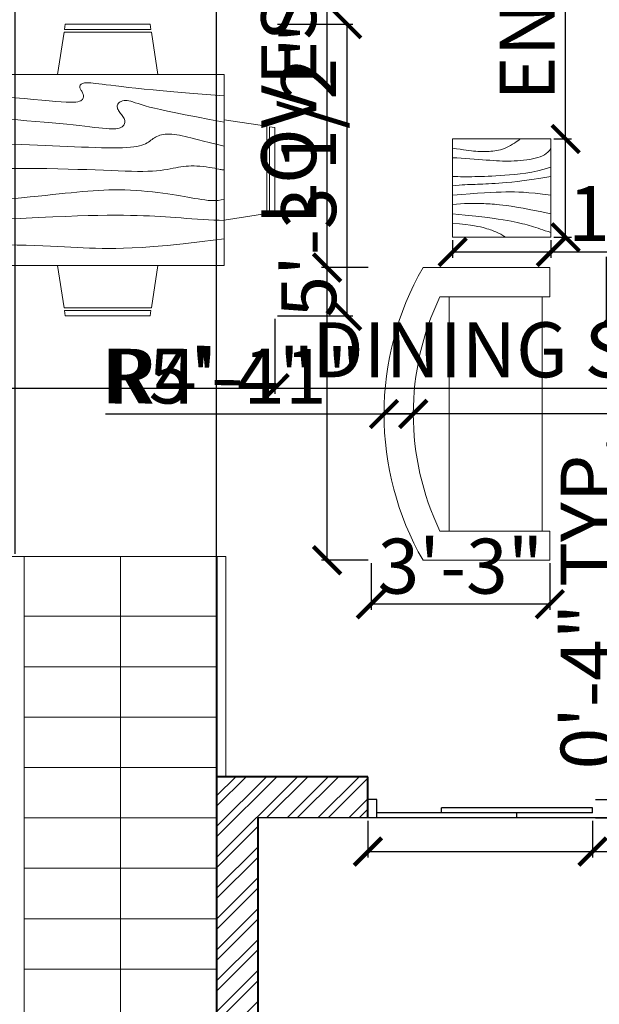
# Model space of a CAD drawing. Units: inches. Extents: x 982 to 1904, y 735 to 1463.
# Tile 4 of 7: x 1439 to 1566, y 945 to 1160. Entities that reach past the tile are written whole.
import ezdxf

# ---------------------------------------------------------------- set-up
doc = ezdxf.new("R2010")
doc.units = ezdxf.units.IN
for name, color, linetype, lineweight in [('A-FLOR', 7, 'Continuous', 25), ('Dimensions', 9, 'Continuous', 18), ('Doors', 130, 'Continuous', 25), ('Furniture', 31, 'Continuous', 18), ('Stairs', 50, 'Continuous', 20), ('Wall Hatch', 23, 'Continuous', 13), ('Walls', 151, 'Continuous', 40)]:
    doc.layers.add(name, color=color, linetype=linetype, lineweight=lineweight)
doc.styles.get("Standard").update_dxf_attribs({"font": 'arial.ttf'})
doc.dimstyles.new('ISO-25', dxfattribs={"dimtxt": 12, "dimasz": 6, "dimexe": 1.25, "dimexo": 0.625, "dimtad": 1, "dimlunit": 3, "dimtxsty": 'Standard', "dimblk": 'ARCHTICK', "dimcen": 2.5, "dimadec": 0, "dimazin": 0, "dimtfac": 1, "dimtmove": 0, "dimatfit": 3, "dimfxl": 1, "dimarcsym": 0})

# ---------------------------------------------------------------- blocks, each defined once
blk = doc.blocks.new('Dining Set - 36 x 72 in.')
for p, q in [((-22.2343, 26.00059), (-23.4847, 17.99762)), ((-22.2304, 26), (-5.7608, 26)), ((-22, 27.5), (-22.1562, 26.50042)), ((-5.8416, 26.5), (-22.1534, 26.5)), ((-22, 27.5), (-6, 27.5)), ((-5.8437, 26.49966), (-6, 27.5)), ((-4.5152, 17.99762), (-5.7655, 25.99926)), ((5.7657, 26.00059), (4.5153, 17.99762)), ((5.7696, 26), (22.2392, 26)), ((6, 27.5), (5.8438, 26.50042)), ((22.1584, 26.5), (5.8466, 26.5)), ((6, 27.5), (22, 27.5)), ((22.1563, 26.49966), (22, 27.5)), ((23.4848, 17.99762), (22.2345, 25.99926)), ((36, 18), (-36, 18)), ((-36, 18), (-36, -18)), ((36, -18), (36, 18)), ((-44.0006, 8.23428), (-35.9976, 9.48474)), ((44.0006, 8.23428), (35.9976, 9.48474)), ((-45.5, 8), (-44.5004, 8.15617)), ((-45.5, 8), (-45.5, -8)), ((-44.5, -8.15843), (-44.5, 8.15338)), ((-44, 8.23041), (-44, -8.23915)), ((44, 8.23041), (44, -8.23915)), ((44.5, -8.15843), (44.5, 8.15338)), ((45.5, 8), (44.5005, 8.15617)), ((45.5, 8), (45.5, -8)), ((-44.4997, -8.15631), (-45.5, -8)), ((-35.9976, -9.48476), (-43.9993, -8.2345)), ((35.9976, -9.48476), (43.9993, -8.2345)), ((44.4997, -8.15631), (45.5, -8)), ((-36, -18), (36, -18)), ((-22.2343, -26.0006), (-23.4847, -17.99762)), ((-4.5152, -17.99762), (-5.7655, -25.99928)), ((5.7657, -26.0006), (4.5153, -17.99762)), ((23.4848, -17.99762), (22.2345, -25.99928)), ((-22.2304, -26), (-5.7608, -26)), ((-22, -27.5), (-22.1562, -26.50044)), ((-5.8416, -26.5), (-22.1534, -26.5)), ((-22, -27.5), (-6, -27.5)), ((-5.8437, -26.49967), (-6, -27.5)), ((5.7696, -26), (22.2392, -26)), ((6, -27.5), (5.8438, -26.50044)), ((22.1584, -26.5), (5.8466, -26.5)), ((6, -27.5), (22, -27.5)), ((22.1563, -26.49967), (22, -27.5))]:
    blk.add_line(p, q)
for points in [[(-36, 15), (-31.1772, 14.97754), (-26.8079, 14.91406), (-22.8538, 14.81543), (-19.276, 14.6875), (-16.0362, 14.53613), (-13.0957, 14.36718), (-10.4159, 14.18652), (-7.9583, 14), (-5.6904, 13.81315), (-3.6035, 13.63021), (-1.6954, 13.45508), (0.0365, 13.29166), (1.5945, 13.14388), (2.9811, 13.01562), (4.1988, 12.9108), (5.25, 12.83333), (6.1393, 12.78613), (6.8802, 12.76823), (7.4883, 12.77767), (7.9792, 12.8125), (8.3685, 12.87077), (8.6719, 12.95052), (8.9049, 13.0498), (9.0833, 13.16666), (9.2205, 13.29899), (9.3216, 13.44401), (9.3895, 13.59879), (9.4271, 13.76041), (9.4373, 13.92594), (9.4232, 14.09245), (9.3875, 14.257), (9.3333, 14.41666), (9.2638, 14.56917), (9.1836, 14.71484), (9.0975, 14.85465), (9.0104, 14.98958), (8.9272, 15.1206), (8.8529, 15.2487), (8.7922, 15.37483), (8.75, 15.5), (8.7305, 15.62467), (8.7344, 15.74739), (8.7617, 15.86621), (8.8125, 15.97916), (8.8867, 16.08431), (8.9844, 16.17968), (9.1055, 16.26334), (9.25, 16.33333), (9.4189, 16.38802), (9.6172, 16.42708), (9.8506, 16.45052), (10.125, 16.45833), (10.4463, 16.45052), (10.8203, 16.42708), (11.2529, 16.38802), (11.75, 16.33333), (12.3184, 16.26318), (12.9694, 16.17838), (13.7151, 16.07991), (14.5677, 15.96875), (15.5395, 15.84586), (16.6426, 15.71224), (17.8893, 15.56884), (19.2917, 15.41666), (20.859, 15.25667), (22.5879, 15.08984), (24.4721, 14.91715), (26.5052, 14.73958), (28.6809, 14.5581), (30.9929, 14.3737), (33.4347, 14.18733), (36, 14)], [(-36, 10), (-28.9766, 10.14274), (-23.1725, 10.20442), (-18.4241, 10.19775), (-14.5677, 10.13541), (-11.4399, 10.03011), (-8.877, 9.89453), (-6.7154, 9.74137), (-4.7917, 9.58333), (-2.9698, 9.43082), (-1.2246, 9.28515), (0.4415, 9.14534), (2.026, 9.01041), (3.5266, 8.87939), (4.9408, 8.7513), (6.266, 8.62516), (7.5, 8.5), (8.6411, 8.37549), (9.6914, 8.2539), (10.6538, 8.13818), (11.5312, 8.03125), (12.3267, 7.93603), (13.043, 7.85547), (13.6831, 7.79248), (14.25, 7.75), (14.7471, 7.7303), (15.1797, 7.73307), (15.5537, 7.75732), (15.875, 7.80208), (16.1494, 7.86637), (16.3828, 7.94922), (16.5811, 8.04964), (16.75, 8.16666), (16.8944, 8.29915), (17.0143, 8.44531), (17.1089, 8.60319), (17.1771, 8.77083), (17.218, 8.94629), (17.2305, 9.1276), (17.2137, 9.31282), (17.1667, 9.5), (17.0895, 9.6875), (16.987, 9.875), (16.8649, 10.0625), (16.7292, 10.25), (16.5856, 10.4375), (16.4401, 10.625), (16.2985, 10.8125), (16.1667, 11), (16.05, 11.18733), (15.9518, 11.3737), (15.8752, 11.5581), (15.8229, 11.73958), (15.798, 11.91715), (15.8034, 12.08984), (15.842, 12.25667), (15.9167, 12.41666), (16.0295, 12.56836), (16.1784, 12.70833), (16.3605, 12.83268), (16.5729, 12.9375), (16.8127, 13.01888), (17.0768, 13.07291), (17.3625, 13.0957), (17.6667, 13.08333), (17.9894, 13.03312), (18.3418, 12.94726), (18.7382, 12.82918), (19.1927, 12.68229), (19.7195, 12.51001), (20.3327, 12.31575), (21.0465, 12.10294), (21.875, 11.875), (22.8357, 11.63354), (23.959, 11.37304), (25.2786, 11.08618), (26.8282, 10.76562), (28.6414, 10.40405), (30.752, 9.99414), (33.1936, 9.52856), (36, 9)], [(-36, 5.5), (-30.7157, 5.3348), (-26.069, 5.20963), (-21.9946, 5.11767), (-18.4271, 5.05208), (-15.3009, 5.00602), (-12.5508, 4.97265), (-10.1112, 4.94515), (-7.9167, 4.91666), (-5.909, 4.88167), (-4.0586, 4.83984), (-2.3429, 4.79215), (-0.7396, 4.73958), (0.7739, 4.6831), (2.22, 4.6237), (3.6213, 4.56233), (5, 4.5), (6.373, 4.43782), (7.7344, 4.3776), (9.0723, 4.32129), (10.375, 4.27083), (11.6309, 4.22819), (12.8281, 4.19531), (13.9551, 4.17415), (15, 4.16666), (15.954, 4.17448), (16.819, 4.19791), (17.6001, 4.23698), (18.3021, 4.29166), (18.9299, 4.36198), (19.4883, 4.44791), (19.9823, 4.54948), (20.4167, 4.66666), (20.7969, 4.79899), (21.1302, 4.94401), (21.4245, 5.09879), (21.6875, 5.26041), (21.9271, 5.42594), (22.1511, 5.59245), (22.3672, 5.757), (22.5834, 5.91666), (22.8065, 6.06868), (23.0404, 6.21093), (23.2879, 6.34147), (23.5521, 6.45833), (23.8358, 6.55957), (24.142, 6.64323), (24.4735, 6.70735), (24.8334, 6.75), (25.2235, 6.76969), (25.642, 6.76692), (26.0858, 6.74267), (26.5521, 6.69791), (27.0379, 6.63362), (27.5404, 6.55078), (28.0565, 6.45036), (28.5834, 6.33333), (29.1242, 6.19987), (29.7071, 6.04687), (30.3661, 5.87044), (31.1354, 5.66666), (32.0493, 5.43164), (33.142, 5.16146), (34.4475, 4.85221), (36, 4.5)], [(-36, -1), (-30.7915, -0.6591), (-26.0195, -0.38216), (-21.6519, -0.16284), (-17.6563, 0.00521), (-14.0005, 0.12833), (-10.6523, 0.21289), (-7.5796, 0.26522), (-4.75, 0.29166), (-2.134, 0.29793), (0.2878, 0.28711), (2.5317, 0.26163), (4.6146, 0.22396), (6.5529, 0.17651), (8.3633, 0.12174), (10.0623, 0.06209), (11.6667, 0), (13.1899, -0.06201), (14.6341, -0.1211), (15.9982, -0.17432), (17.2813, -0.21875), (18.4823, -0.25147), (19.6003, -0.26953), (20.6343, -0.27002), (21.5834, -0.25), (22.4481, -0.20768), (23.2357, -0.14584), (23.9549, -0.06836), (24.6146, 0.02083), (25.2235, 0.11784), (25.7904, 0.21875), (26.3241, 0.31966), (26.8334, 0.41666), (27.3265, 0.50618), (27.8099, 0.58593), (28.2894, 0.65397), (28.7709, 0.70833), (29.2601, 0.74707), (29.763, 0.76823), (30.2855, 0.76985), (30.8334, 0.75), (31.4088, 0.70784), (31.9994, 0.64713), (32.589, 0.57275), (33.1615, 0.48958), (33.7008, 0.4025), (34.1908, 0.3164), (34.6153, 0.23616), (34.9584, 0.16666), (35.2099, 0.11165), (35.3848, 0.07031), (35.504, 0.04069), (35.5886, 0.02083), (35.6594, 0.00879), (35.7377, 0.0026), (35.8442, 0.00032), (36, 0)], [(-36, -6.5), (-27.1843, -6.31267), (-20.084, -6.1263), (-14.469, -5.9419), (-10.1094, -5.76042), (-6.7752, -5.58285), (-4.2363, -5.41016), (-2.2629, -5.24333), (-0.625, -5.08334), (0.8708, -4.93099), (2.2715, -4.78646), (3.5872, -4.64974), (4.8281, -4.52084), (6.0046, -4.39974), (7.127, -4.28646), (8.2053, -4.18099), (9.25, -4.08334), (10.2705, -3.99382), (11.2734, -3.91407), (12.2647, -3.84603), (13.25, -3.79167), (14.2354, -3.75293), (15.2266, -3.73177), (16.2295, -3.73015), (17.25, -3.75), (18.2912, -3.79248), (19.3451, -3.85547), (20.4009, -3.93604), (21.4479, -4.03125), (22.4754, -4.13819), (23.4727, -4.25391), (24.4289, -4.37549), (25.3334, -4.5), (26.1785, -4.62492), (26.9694, -4.74935), (27.7145, -4.87281), (28.4219, -4.99479), (29.1, -5.11483), (29.7572, -5.23242), (30.4016, -5.34709), (31.0417, -5.45834), (31.6837, -5.56437), (32.3262, -5.65821), (32.9658, -5.73153), (33.599, -5.77604), (34.2224, -5.78345), (34.8327, -5.74545), (35.4264, -5.65373), (36, -5.5)], [(-36, -10), (-26.4022, -9.81299), (-18.4675, -9.62891), (-11.9839, -9.45069), (-6.7396, -9.28125), (-2.5226, -9.12354), (0.8789, -8.98047), (3.6769, -8.85498), (6.0833, -8.75), (8.2767, -8.66765), (10.3021, -8.60677), (12.1712, -8.56543), (13.8958, -8.54167), (15.4876, -8.53353), (16.9583, -8.53907), (18.3197, -8.55632), (19.5834, -8.58334), (20.7616, -8.61841), (21.8685, -8.66081), (22.9188, -8.71004), (23.9271, -8.76563), (24.9081, -8.82707), (25.8763, -8.89388), (26.8465, -8.96558), (27.8334, -9.04167), (28.8474, -9.12118), (29.8828, -9.20117), (30.93, -9.27824), (31.9792, -9.34896), (33.0205, -9.40991), (34.0443, -9.45768), (35.0407, -9.48885), (36, -9.5)], [(-36, -14.5), (-30.0881, -14.33513), (-25.0332, -14.21224), (-20.7312, -14.12647), (-17.0781, -14.07292), (-13.97, -14.04671), (-11.3027, -14.04297), (-8.9724, -14.05681), (-6.875, -14.08334), (-4.9224, -14.11833), (-3.0905, -14.16016), (-1.3709, -14.20785), (0.2448, -14.26042), (1.7647, -14.3169), (3.1973, -14.3763), (4.5507, -14.43767), (5.8333, -14.5), (7.0554, -14.5621), (8.235, -14.62175), (9.3922, -14.67652), (10.5469, -14.72396), (11.7192, -14.76164), (12.929, -14.78711), (14.1965, -14.79794), (15.5417, -14.79167), (16.9933, -14.76424), (18.6152, -14.70508), (20.4804, -14.60197), (22.6615, -14.44271), (25.2312, -14.21509), (28.2624, -13.9069), (31.8277, -13.50594), (36, -13)]]:
    blk.add_lwpolyline(points)
blk = doc.blocks.new('Sofa - Roundback Loveseat 5 ft.')
for p, q in [((0, -32.44198), (0, -5.99998)), ((-24, -33.99998), (-24, -11.46958)), ((24.00004, -33.99998), (24.00004, -11.46958)), ((-23.9998, -13.38178), (23.99986, -13.38178)), ((-24, -32.44198), (24.00004, -32.44198))]:
    blk.add_line(p, q)
for points in [[(-24, -33.99998), (-30, -33.99998), (-30, -7.99998)], [(30.00004, -7.99998), (30.00004, -33.99998), (24.00004, -33.99998)]]:
    blk.add_lwpolyline(points)
for centre, radius, start, end in [((0, -60.24998), 60.24998, 60.13715, 119.8628), ((0, -61.38438), 55.38444, 64.32083, 115.6792)]:
    blk.add_arc(centre, radius, start, end)
blk = doc.blocks.new('Table - Square Woodgrain 42 x 42 in.')
blk.add_line((0, -42), (42, -42))
for points in [[(0, -4), (1.704, -4.2172), (3.2358, -4.4188), (4.615, -4.604), (5.8615, -4.7721), (6.9951, -4.9224), (8.0357, -5.0541), (9.0031, -5.1667), (9.9171, -5.2594), (10.7951, -5.3316), (11.6445, -5.3836), (12.4702, -5.4157), (13.277, -5.4283), (14.0698, -5.4217), (14.8535, -5.3964), (15.6331, -5.3526), (16.4133, -5.2908), (17.1986, -5.2103), (17.9913, -5.1062), (18.793, -4.9727), (19.6056, -4.8038), (20.4307, -4.5937), (21.2701, -4.3365), (22.1256, -4.0262), (22.9989, -3.6571), (23.888, -3.2272), (24.7756, -2.7516), (25.6408, -2.2491), (26.4624, -1.7387), (27.2195, -1.2395), (27.891, -0.7703), (28.456, -0.3501), (28.8934, 0.002)], [(0, -42), (0, 0), (42, 0), (42, -42)], [(0, -8), (1.8203, -8.1001), (3.6741, -8.2149), (5.5411, -8.3408), (7.4011, -8.4741), (9.2339, -8.6112), (11.0193, -8.7484), (12.7371, -8.8821), (14.3671, -9.0086), (15.8954, -9.1246), (17.3337, -9.2278), (18.6997, -9.3159), (20.0116, -9.387), (21.2871, -9.4389), (22.5442, -9.4696), (23.8008, -9.477), (25.0749, -9.459), (26.3791, -9.4137), (27.7049, -9.3403), (29.0383, -9.2382), (30.3655, -9.1068), (31.6728, -8.9455), (32.9461, -8.7535), (34.1717, -8.5304), (35.3358, -8.2756), (36.4268, -7.9863), (37.443, -7.6521), (38.3849, -7.2603), (39.253, -6.7986), (40.048, -6.2542), (40.7705, -5.6147), (41.421, -4.8674), (42, -4)], [(42, -12), (39.1784, -12.8621), (36.4519, -13.5654), (33.8246, -14.1294), (31.3004, -14.5731), (28.8832, -14.9161), (26.577, -15.1775), (24.3858, -15.3768), (22.3136, -15.5332), (20.3622, -15.6632), (18.5254, -15.7718), (16.7947, -15.8612), (15.1618, -15.9338), (13.6183, -15.9916), (12.1558, -16.0369), (10.7659, -16.0718), (9.4403, -16.0987), (8.1703, -16.1191), (6.9461, -16.1325), (5.7577, -16.1377), (4.595, -16.1335), (3.4479, -16.1188), (2.3064, -16.0924), (1.1604, -16.0532), (0, -16)], [(42, -16), (37.6529, -16.7365), (33.8802, -17.329), (30.6179, -17.7961), (27.8015, -18.1561), (25.3668, -18.4275), (23.2497, -18.6288), (21.3859, -18.7785), (19.7111, -18.8949), (18.1693, -18.9939), (16.7375, -19.0795), (15.401, -19.1534), (14.1449, -19.217), (12.9544, -19.2717), (11.8148, -19.3191), (10.7113, -19.3606), (9.6291, -19.3976), (8.5534, -19.4323), (7.47, -19.4689), (6.3643, -19.5122), (5.222, -19.5672), (4.0288, -19.6386), (2.7703, -19.7313), (1.4321, -19.8501), (0, -20)], [(0, -24), (3.9243, -23.6805), (7.4766, -23.4138), (10.6891, -23.1954), (13.5943, -23.0205), (16.2247, -22.8847), (18.6125, -22.7832), (20.7903, -22.7116), (22.7903, -22.6651), (24.6563, -22.642), (26.4764, -22.6507), (28.35, -22.7024), (30.3766, -22.8084), (32.6555, -22.98), (35.2861, -23.2283), (38.3678, -23.5645), (42, -24)], [(42, -32), (37.392, -31.017), (33.4585, -30.2231), (30.1291, -29.5949), (27.3334, -29.109), (25.0009, -28.742), (23.0612, -28.4707), (21.4439, -28.2716), (20.0786, -28.1215), (18.8998, -28.0002), (17.8609, -27.9014), (16.9206, -27.8219), (16.0371, -27.7588), (15.1691, -27.709), (14.2748, -27.6693), (13.3128, -27.6368), (12.2415, -27.6083), (11.0295, -27.5824), (9.6867, -27.5643), (8.233, -27.5608), (6.6884, -27.5787), (5.0728, -27.6248), (3.4062, -27.7058), (1.7086, -27.8286), (0, -28)], [(0, -32), (5.4026, -32.5358), (9.9494, -33.019), (13.7424, -33.4553), (16.8834, -33.8505), (19.4743, -34.2106), (21.6171, -34.5413), (23.4136, -34.8486), (24.9657, -35.1382), (26.3614, -35.4156), (27.6332, -35.6841), (28.7995, -35.9467), (29.8788, -36.2064), (30.8897, -36.4661), (31.8507, -36.7288), (32.7802, -36.9973), (33.6968, -37.2747), (34.6175, -37.5635), (35.5531, -37.8651), (36.5128, -38.1805), (37.506, -38.5108), (38.5421, -38.8568), (39.6302, -39.2197), (40.7797, -39.6004), (42, -40)], [(0, -36), (3.0098, -36.2857), (5.5354, -36.5643), (7.6368, -36.8359), (9.374, -37.1009), (10.807, -37.3597), (11.9957, -37.6126), (13.0002, -37.8599), (13.8804, -38.102), (14.6874, -38.3393), (15.4365, -38.5729), (16.1338, -38.8041), (16.7858, -39.0341), (17.3987, -39.264), (17.9787, -39.4952), (18.5322, -39.7288), (19.0655, -39.9662), (19.5832, -40.2081), (20.0842, -40.4544), (20.5657, -40.7046), (21.0249, -40.9581), (21.459, -41.2144), (21.8653, -41.4731), (22.2409, -41.7335), (22.5831, -41.9951)]]:
    blk.add_lwpolyline(points)
blk = doc.blocks.new('DOOR-SLIDING-PANEL')
for p, q in [((2, 4), (0, 4)), ((2, 0), (2, 4)), ((49.05, 2.21), (16.06, 2.21)), ((16.06, 1.11), (16.06, 2.21)), ((49.05, 1.11), (49.05, 2.21)), ((49.05, 1.11), (2, 1.11)), ((32.55, 0), (32.55, 1.11))]:
    blk.add_line(p, q)
blk = doc.blocks.new('_ArchTick')
at = {"color": 0, "linetype": 'ByBlock', "const_width": 0.15}
blk.add_lwpolyline([(-0.5, -0.5), (0.5, 0.5)], dxfattribs=at)
blk = doc.blocks.new('*D38')
at = {"layer": 'Defpoints', "color": 0, "transparency": 16777216}
for p in [(1515.5, 985.99), (1564.55, 985.99), (1564.55, 978.63)]:
    blk.add_point(p, dxfattribs=at)
at = {"layer": 'Dimensions', "color": 0, "lineweight": -2, "transparency": 16777216}
for p, q in [((1515.5, 985.37), (1515.5, 977.38)), ((1564.55, 985.37), (1564.55, 977.38)), ((1515.5, 978.63), (1564.55, 978.63)), ((1564.55, 978.63), (1776.25, 978.63))]:
    blk.add_line(p, q, dxfattribs=at)
at = {"layer": 'Dimensions', "color": 0, "lineweight": -2, "transparency": 16777216, "xscale": 6, "yscale": 6, "zscale": 6, "rotation": 180}
blk.add_blockref('_ArchTick', (1515.5, 978.63), dxfattribs=at)
at = {"layer": 'Dimensions', "color": 0, "lineweight": -2, "transparency": 16777216, "xscale": 6, "yscale": 6, "zscale": 6}
blk.add_blockref('_ArchTick', (1564.55, 978.63), dxfattribs=at)
at = {"layer": 'Dimensions', "color": 0, "transparency": 16777216, "insert": (1673.4, 985.46), "char_height": 12, "attachment_point": 5}
blk.add_mtext('SLIDING PANEL 4\'-1" TYP.', dxfattribs=at)
blk = doc.blocks.new('*D39')
at = {"layer": 'Defpoints', "color": 0, "transparency": 16777216}
for p in [(1564.55, 989.99), (1571.9, 989.99), (1564.55, 985.99)]:
    blk.add_point(p, dxfattribs=at)
at = {"layer": 'Dimensions', "color": 0, "lineweight": -2, "transparency": 16777216}
for p, q in [((1571.9, 989.99), (1571.9, 1070.39)), ((1565.17, 989.99), (1573.15, 989.99)), ((1571.9, 985.99), (1571.9, 989.99)), ((1565.17, 985.99), (1573.15, 985.99))]:
    blk.add_line(p, q, dxfattribs=at)
at = {"layer": 'Dimensions', "color": 0, "lineweight": -2, "transparency": 16777216, "xscale": 6, "yscale": 6, "zscale": 6}
for p, rotation in [((1571.9, 989.99), 90), ((1571.9, 985.99), 270)]:
    blk.add_blockref('_ArchTick', p, dxfattribs=dict(at, rotation=rotation))
at = {"layer": 'Dimensions', "color": 0, "transparency": 16777216, "insert": (1565.15, 1033.19), "char_height": 12, "attachment_point": 5, "rotation": 90}
blk.add_mtext('0\'-4" TYP.', dxfattribs=at)
blk = doc.blocks.new('*D40')
at = {"layer": 'Defpoints', "color": 0, "transparency": 16777216}
for p in [(1389.84, 1095.57), (1495.17, 1095.57), (1495.17, 1079.77)]:
    blk.add_point(p, dxfattribs=at)
at = {"layer": 'Dimensions', "color": 0, "lineweight": -2, "transparency": 16777216}
for p, q in [((1389.84, 1094.94), (1389.84, 1078.52)), ((1495.17, 1094.94), (1495.17, 1078.52)), ((1389.84, 1079.77), (1495.17, 1079.77)), ((1495.17, 1079.77), (1662.27, 1079.77))]:
    blk.add_line(p, q, dxfattribs=at)
at = {"layer": 'Dimensions', "color": 0, "lineweight": -2, "transparency": 16777216, "xscale": 6, "yscale": 6, "zscale": 6, "rotation": 180}
blk.add_blockref('_ArchTick', (1389.84, 1079.77), dxfattribs=at)
at = {"layer": 'Dimensions', "color": 0, "lineweight": -2, "transparency": 16777216, "xscale": 6, "yscale": 6, "zscale": 6}
blk.add_blockref('_ArchTick', (1495.17, 1079.77), dxfattribs=at)
at = {"layer": 'Dimensions', "color": 0, "transparency": 16777216, "insert": (1581.72, 1086.6), "char_height": 12, "attachment_point": 5}
blk.add_mtext('DINING SET 8\'-9 1/2"', dxfattribs=at)
blk = doc.blocks.new('*D41')
at = {"layer": 'Defpoints', "color": 0, "transparency": 16777216}
for p in [(1495.17, 1159.23), (1510.97, 1159.23), (1495.17, 1095.57)]:
    blk.add_point(p, dxfattribs=at)
at = {"layer": 'Dimensions', "color": 0, "lineweight": -2, "transparency": 16777216}
for p, q in [((1495.79, 1159.23), (1512.22, 1159.23)), ((1510.97, 1095.57), (1510.97, 1159.23)), ((1495.79, 1095.57), (1512.22, 1095.57))]:
    blk.add_line(p, q, dxfattribs=at)
at = {"layer": 'Dimensions', "color": 0, "lineweight": -2, "transparency": 16777216, "xscale": 6, "yscale": 6, "zscale": 6}
for p, rotation in [((1510.97, 1159.23), 90), ((1510.97, 1095.57), 270)]:
    blk.add_blockref('_ArchTick', p, dxfattribs=dict(at, rotation=rotation))
at = {"layer": 'Dimensions', "color": 0, "transparency": 16777216, "insert": (1504.14, 1127.4), "char_height": 12, "attachment_point": 5, "rotation": 90}
blk.add_mtext('5\'-3 1/2"', dxfattribs=at)
blk = doc.blocks.new('*D42')
at = {"layer": 'Defpoints', "color": 0, "transparency": 16777216}
for p in [(1567.53, 1109.05), (1666.29, 1109.05), (1666.29, 1094.24)]:
    blk.add_point(p, dxfattribs=at)
at = {"layer": 'Dimensions', "color": 0, "lineweight": -2, "transparency": 16777216}
for p, q in [((1567.53, 1108.43), (1567.53, 1092.99)), ((1666.29, 1108.43), (1666.29, 1092.99)), ((1567.53, 1094.24), (1666.29, 1094.24))]:
    blk.add_line(p, q, dxfattribs=at)
at = {"layer": 'Dimensions', "color": 0, "lineweight": -2, "transparency": 16777216, "xscale": 6, "yscale": 6, "zscale": 6, "rotation": 180}
blk.add_blockref('_ArchTick', (1567.53, 1094.24), dxfattribs=at)
at = {"layer": 'Dimensions', "color": 0, "lineweight": -2, "transparency": 16777216, "xscale": 6, "yscale": 6, "zscale": 6}
blk.add_blockref('_ArchTick', (1666.29, 1094.24), dxfattribs=at)
at = {"layer": 'Dimensions', "color": 0, "transparency": 16777216, "insert": (1616.91, 1101.08), "char_height": 12, "attachment_point": 5}
blk.add_mtext('SOFA 8\'-3"', dxfattribs=at)
blk = doc.blocks.new('*D44')
at = {"layer": 'Defpoints', "color": 0, "transparency": 16777216}
for p in [(1506.61, 1106.1), (1516.2, 1106.1), (1516.2, 1042.21)]:
    blk.add_point(p, dxfattribs=at)
at = {"layer": 'Dimensions', "color": 0, "lineweight": -2, "transparency": 16777216}
for p, q in [((1506.61, 1106.1), (1506.61, 1237.89)), ((1515.57, 1106.1), (1505.36, 1106.1)), ((1506.61, 1042.21), (1506.61, 1106.1)), ((1515.57, 1042.21), (1505.36, 1042.21))]:
    blk.add_line(p, q, dxfattribs=at)
at = {"layer": 'Dimensions', "color": 0, "lineweight": -2, "transparency": 16777216, "xscale": 6, "yscale": 6, "zscale": 6}
for p, rotation in [((1506.61, 1106.1), 90), ((1506.61, 1042.21), 270)]:
    blk.add_blockref('_ArchTick', p, dxfattribs=dict(at, rotation=rotation))
at = {"layer": 'Dimensions', "color": 0, "transparency": 16777216, "insert": (1499.78, 1175), "char_height": 12, "attachment_point": 5, "rotation": 90}
blk.add_mtext('LOVESEAT 5\'-4"', dxfattribs=at)
blk = doc.blocks.new('*D45')
at = {"layer": 'Defpoints', "color": 0, "transparency": 16777216}
for p in [(1516.2, 1042.21), (1555.24, 1042.21), (1516.2, 1032.63)]:
    blk.add_point(p, dxfattribs=at)
at = {"layer": 'Dimensions', "color": 0, "lineweight": -2, "transparency": 16777216}
for p, q in [((1516.2, 1041.58), (1516.2, 1031.38)), ((1555.24, 1041.58), (1555.24, 1031.38)), ((1555.24, 1032.63), (1516.2, 1032.63))]:
    blk.add_line(p, q, dxfattribs=at)
at = {"layer": 'Dimensions', "color": 0, "lineweight": -2, "transparency": 16777216, "xscale": 6, "yscale": 6, "zscale": 6, "rotation": 180}
blk.add_blockref('_ArchTick', (1516.2, 1032.63), dxfattribs=at)
at = {"layer": 'Dimensions', "color": 0, "lineweight": -2, "transparency": 16777216, "xscale": 6, "yscale": 6, "zscale": 6}
blk.add_blockref('_ArchTick', (1555.24, 1032.63), dxfattribs=at)
at = {"layer": 'Dimensions', "color": 0, "transparency": 16777216, "insert": (1535.72, 1039.38), "char_height": 12, "attachment_point": 5}
blk.add_mtext('3\'-3"', dxfattribs=at)
blk = doc.blocks.new('*D48')
at = {"layer": 'Defpoints', "color": 0, "transparency": 16777216}
for p in [(1555.46, 1134.17), (1558.68, 1134.17), (1555.46, 1112.72)]:
    blk.add_point(p, dxfattribs=at)
at = {"layer": 'Dimensions', "color": 0, "lineweight": -2, "transparency": 16777216}
for p, q in [((1558.68, 1134.17), (1558.68, 1298.47)), ((1556.09, 1134.17), (1559.93, 1134.17)), ((1558.68, 1112.72), (1558.68, 1134.17)), ((1556.09, 1112.72), (1559.93, 1112.72))]:
    blk.add_line(p, q, dxfattribs=at)
at = {"layer": 'Dimensions', "color": 0, "lineweight": -2, "transparency": 16777216, "xscale": 6, "yscale": 6, "zscale": 6}
for p, rotation in [((1558.68, 1134.17), 90), ((1558.68, 1112.72), 270)]:
    blk.add_blockref('_ArchTick', p, dxfattribs=dict(at, rotation=rotation))
at = {"layer": 'Dimensions', "color": 0, "transparency": 16777216, "insert": (1551.85, 1219.32), "char_height": 12, "attachment_point": 5, "rotation": 90}
blk.add_mtext('END TABLE 1\'-9 1/2"', dxfattribs=at)
blk = doc.blocks.new('*D49')
at = {"layer": 'Defpoints', "color": 0, "transparency": 16777216}
for p in [(1534.01, 1112.72), (1555.46, 1112.72), (1555.46, 1109.5)]:
    blk.add_point(p, dxfattribs=at)
at = {"layer": 'Dimensions', "color": 0, "lineweight": -2, "transparency": 16777216}
for p, q in [((1534.01, 1112.09), (1534.01, 1108.25)), ((1555.46, 1112.09), (1555.46, 1108.25)), ((1534.01, 1109.5), (1555.46, 1109.5)), ((1555.46, 1109.5), (1621.44, 1109.5))]:
    blk.add_line(p, q, dxfattribs=at)
at = {"layer": 'Dimensions', "color": 0, "lineweight": -2, "transparency": 16777216, "xscale": 6, "yscale": 6, "zscale": 6, "rotation": 180}
blk.add_blockref('_ArchTick', (1534.01, 1109.5), dxfattribs=at)
at = {"layer": 'Dimensions', "color": 0, "lineweight": -2, "transparency": 16777216, "xscale": 6, "yscale": 6, "zscale": 6}
blk.add_blockref('_ArchTick', (1555.46, 1109.5), dxfattribs=at)
at = {"layer": 'Dimensions', "color": 0, "transparency": 16777216, "insert": (1591.45, 1116.33), "char_height": 12, "attachment_point": 5}
blk.add_mtext('1\'-9 1/2"', dxfattribs=at)
blk = doc.blocks.new('*D64')
at = {"layer": 'Defpoints', "color": 0, "transparency": 16777216}
for p in [(1482.5, 1427.79), (1370.5, 841.99), (1482.5, 841.99)]:
    blk.add_point(p, dxfattribs=at)
at = {"layer": 'Dimensions', "color": 0, "lineweight": -2, "transparency": 16777216}
for p, q in [((1370.5, 842.62), (1370.5, 1429.04)), ((1482.5, 842.62), (1482.5, 1429.04)), ((1370.5, 1427.79), (1482.5, 1427.79))]:
    blk.add_line(p, q, dxfattribs=at)
at = {"layer": 'Dimensions', "color": 0, "lineweight": -2, "transparency": 16777216, "xscale": 6, "yscale": 6, "zscale": 6, "rotation": 180}
blk.add_blockref('_ArchTick', (1370.5, 1427.79), dxfattribs=at)
at = {"layer": 'Dimensions', "color": 0, "lineweight": -2, "transparency": 16777216, "xscale": 6, "yscale": 6, "zscale": 6}
blk.add_blockref('_ArchTick', (1482.5, 1427.79), dxfattribs=at)
at = {"layer": 'Dimensions', "color": 0, "transparency": 16777216, "insert": (1426.5, 1434.54), "char_height": 12, "attachment_point": 5}
blk.add_mtext('9\'-4"', dxfattribs=at)
blk = doc.blocks.new('*D66')
at = {"layer": 'Defpoints', "color": 0, "transparency": 16777216}
for p in [(1482.5, 1427.79), (1438.5, 1043.01), (1482.5, 1043.03)]:
    blk.add_point(p, dxfattribs=at)
at = {"layer": 'Dimensions', "color": 0, "lineweight": -2, "transparency": 16777216}
for p, q in [((1438.5, 1043.64), (1438.5, 1429.04)), ((1482.5, 1043.65), (1482.5, 1429.04)), ((1438.5, 1427.79), (1482.5, 1427.79))]:
    blk.add_line(p, q, dxfattribs=at)
at = {"layer": 'Dimensions', "color": 0, "lineweight": -2, "transparency": 16777216, "xscale": 6, "yscale": 6, "zscale": 6, "rotation": 180}
blk.add_blockref('_ArchTick', (1438.5, 1427.79), dxfattribs=at)
at = {"layer": 'Dimensions', "color": 0, "lineweight": -2, "transparency": 16777216, "xscale": 6, "yscale": 6, "zscale": 6}
blk.add_blockref('_ArchTick', (1482.5, 1427.79), dxfattribs=at)
at = {"layer": 'Dimensions', "color": 0, "transparency": 16777216, "insert": (1460.5, 1434.55), "char_height": 12, "attachment_point": 5}
blk.add_mtext('3\'-8"', dxfattribs=at)
blk = doc.blocks.new('*D76')
at = {"layer": 'Defpoints', "color": 0, "transparency": 16777216}
for p in [(1519.04, 1074.16), (1583.2, 1074.16)]:
    blk.add_point(p, dxfattribs=at)
at = {"layer": 'Dimensions', "color": 0, "lineweight": -2, "transparency": 16777216}
for p in [(1458.22, 1074.16), (1583.2, 1074.16)]:
    blk.add_line(p, (1519.04, 1074.16), dxfattribs=at)
at = {"layer": 'Dimensions', "color": 0, "lineweight": -2, "transparency": 16777216, "xscale": 6, "yscale": 6, "zscale": 6, "rotation": 359.9995481306522}
blk.add_blockref('_ArchTick', (1519.04, 1074.16), dxfattribs=at)
at = {"layer": 'Dimensions', "color": 0, "transparency": 16777216, "insert": (1480.54, 1080.88), "char_height": 12, "attachment_point": 5, "rotation": 359.9995}
blk.add_mtext('R5\'-4"', dxfattribs=at)
blk = doc.blocks.new('*D77')
at = {"layer": 'Defpoints', "color": 0, "transparency": 16777216}
for p in [(1525.43, 1074.16), (1584.4, 1074.16)]:
    blk.add_point(p, dxfattribs=at)
at = {"layer": 'Dimensions', "color": 0, "lineweight": -2, "transparency": 16777216}
for p in [(1459.47, 1074.16), (1584.4, 1074.16)]:
    blk.add_line(p, (1525.43, 1074.16), dxfattribs=at)
at = {"layer": 'Dimensions', "color": 0, "lineweight": -2, "transparency": 16777216, "xscale": 6, "yscale": 6, "zscale": 6, "rotation": 0.0004799085174027}
blk.add_blockref('_ArchTick', (1525.43, 1074.16), dxfattribs=at)
at = {"layer": 'Dimensions', "color": 0, "transparency": 16777216, "insert": (1486.45, 1080.81), "char_height": 12, "attachment_point": 5, "rotation": 0.0005}
blk.add_mtext('R4\'-11"', dxfattribs=at)

msp = doc.modelspace()

# ---------------------------------------------------------------- hatches: boundary and pattern name
at = {"layer": 'Wall Hatch'}
h = msp.add_hatch(dxfattribs=at)
h.set_pattern_fill('ANSI32', color=256, scale=0.5)
h.paths.add_polyline_path([(1165.496, 1065.991), (1271.496, 1065.991), (1271.496, 1071.991), (1218.496, 1071.991), (1218.496, 1238.491), (1262.496, 1238.491), (1262.496, 1244.491), (1218.496, 1244.491), (1218.496, 1330.491), (1298.496, 1330.491), (1298.496, 1244.491), (1292.496, 1244.491), (1292.496, 1238.491), (1298.496, 1238.491), (1298.496, 1221.991), (1304.496, 1221.991), (1304.496, 1224.991), (1374.496, 1224.991), (1374.496, 1230.991), (1304.496, 1230.991), (1304.496, 1251.991), (1310.496, 1251.991), (1310.496, 1257.991), (1304.496, 1257.991), (1304.496, 1385.991), (1328.496, 1385.991), (1328.496, 1394.991), (1295.496, 1394.991), (1295.496, 1339.491), (1209.496, 1339.491), (1209.496, 1071.991), (1156.496, 1071.991), (1156.496, 893.991), (1171.496, 893.991), (1171.496, 902.991), (1165.496, 902.991)])
h.paths.add_polyline_path([(1273.996, 877.991), (1267.996, 877.991), (1267.996, 902.991), (1252.996, 902.991), (1252.996, 893.991), (1258.996, 893.991), (1258.996, 868.991), (1273.996, 868.991)])
h.paths.add_polyline_path([(1370.496, 1052.991), (1361.496, 1052.991), (1361.496, 1046.991), (1355.496, 1046.991), (1355.496, 1040.991), (1361.496, 1040.991), (1361.496, 877.991), (1355.496, 877.991), (1355.496, 868.991), (1361.496, 868.991), (1361.496, 832.991), (1376.313, 832.991), (1491.496, 832.991), (1491.496, 985.991), (1515.496, 985.991), (1515.496, 994.991), (1482.496, 994.991), (1482.496, 841.991), (1370.496, 841.991)])
h.paths.add_polyline_path([(1319.496, 1088.991), (1325.496, 1088.991), (1325.496, 1094.991), (1319.496, 1094.991), (1319.496, 1112.491), (1361.496, 1112.491), (1361.496, 1094.991), (1355.496, 1094.991), (1355.496, 1088.991), (1361.496, 1088.991), (1361.496, 1082.991), (1370.496, 1082.991), (1370.496, 1180.991), (1503.496, 1180.991), (1503.496, 1231.991), (1497.496, 1231.991), (1497.496, 1215.991), (1491.496, 1215.991), (1491.496, 1209.991), (1497.496, 1209.991), (1497.496, 1189.991), (1448.496, 1189.991), (1448.496, 1209.991), (1454.496, 1209.991), (1454.496, 1215.991), (1448.496, 1215.991), (1448.496, 1221.991), (1442.496, 1221.991), (1442.496, 1189.991), (1380.496, 1189.991), (1380.496, 1251.991), (1442.496, 1251.991), (1442.496, 1245.991), (1448.496, 1245.991), (1448.496, 1263.991), (1442.496, 1263.991), (1442.496, 1257.991), (1368.496, 1257.991), (1368.496, 1251.991), (1374.496, 1251.991), (1374.496, 1189.991), (1304.496, 1189.991), (1304.496, 1192.991), (1295.496, 1192.991), (1295.496, 1183.991), (1361.496, 1183.991), (1361.496, 1118.491), (1313.496, 1118.491), (1313.496, 1071.991), (1301.496, 1071.991), (1301.496, 1065.991), (1313.496, 1065.991), (1313.496, 1040.991), (1325.496, 1040.991), (1325.496, 1046.991), (1319.496, 1046.991)])
h.paths.add_polyline_path([(1565.496, 1394.991), (1418.496, 1394.991), (1418.496, 1385.991), (1442.496, 1385.991), (1442.496, 1293.991), (1448.496, 1293.991), (1448.496, 1299.991), (1454.496, 1299.991), (1454.496, 1305.991), (1448.496, 1305.991), (1448.496, 1385.991), (1556.496, 1385.991), (1556.496, 1307.991), (1497.496, 1307.991), (1497.496, 1305.991), (1491.496, 1305.991), (1491.496, 1299.991), (1497.496, 1299.991), (1497.496, 1268.991), (1503.496, 1268.991), (1503.496, 1298.991), (1656.496, 1298.991), (1656.496, 1307.991), (1565.496, 1307.991)])
h.paths.add_polyline_path([(1731.496, 1307.991), (1698.496, 1307.991), (1698.496, 1298.991), (1722.496, 1298.991), (1722.496, 1033.991), (1731.496, 1033.991)])
h.paths.add_polyline_path([(1731.496, 997.991), (1722.496, 997.991), (1722.496, 994.991), (1689.496, 994.991), (1689.496, 985.991), (1731.496, 985.991)])

# ---------------------------------------------------------------- linework, layer by layer
at = {"layer": 'A-FLOR'}
msp.add_line((1732.746, 985.991), (1491.496, 985.991), dxfattribs=at)
at = {"layer": 'Stairs'}
for p, q in [((1370.496, 1042.991), (1484.496, 1043.026)), ((1440.496, 1043.012), (1440.496, 886.991)), ((1461.496, 886.991), (1461.496, 1043.019)), ((1484.496, 1043.026), (1484.496, 994.991)), ((1440.496, 1029.991), (1482.496, 1029.991)), ((1440.496, 1018.991), (1482.496, 1018.991)), ((1440.496, 1007.991), (1482.496, 1007.991)), ((1440.496, 996.991), (1482.496, 996.991)), ((1440.496, 985.991), (1482.496, 985.991)), ((1440.496, 974.991), (1482.496, 974.991)), ((1440.496, 963.991), (1482.496, 963.991)), ((1440.496, 952.991), (1482.496, 952.991))]:
    msp.add_line(p, q, dxfattribs=at)
at = {"layer": 'Walls'}
for p, q in [((1482.496, 1043.025), (1482.496, 841.991)), ((1515.496, 994.991), (1482.496, 994.991)), ((1515.496, 985.991), (1515.496, 994.991)), ((1491.496, 985.991), (1491.496, 814.991))]:
    msp.add_line(p, q, dxfattribs=at)

# ---------------------------------------------------------------- block references
at = {"layer": 'Doors'}
msp.add_blockref('DOOR-SLIDING-PANEL', (1515.496, 985.991), dxfattribs=at)
at = {"layer": 'Furniture'}
for name, p, xscale, yscale, zscale in [('Dining Set - 36 x 72 in.', (1442.505, 1127.4), 1.157465785560688, 1.157465785560688, 1.157465785560688), ('Table - Square Woodgrain 42 x 42 in.', (1534.008, 1134.172), 0.5107591657752469, 0.5107591657752469, 0.5107591657752469)]:
    msp.add_blockref(name, p, dxfattribs=dict(at, xscale=xscale, yscale=yscale, zscale=zscale))
at = {"layer": 'Furniture', "xscale": 1.064886596901886, "yscale": 1.064886596901886, "zscale": 1.064886596901886, "rotation": 90}
msp.add_blockref('Sofa - Roundback Loveseat 5 ft.', (1519.036, 1074.156), dxfattribs=at)

# ---------------------------------------------------------------- dimensions: what is measured, and where the dimension line sits
at = {"layer": 'Dimensions'}
for base, p1, p2, picture, middle in [((1482.496, 1427.791), (1370.496, 841.991), (1482.496, 841.991), '*D64', (1426.496, 1434.543)), ((1482.496, 1427.791), (1438.496, 1043.012), (1482.496, 1043.025), '*D66', (1460.496, 1434.547)), ((1555.46, 1109.502), (1534.008, 1112.72), (1555.46, 1112.72), '*D49', (1591.451, 1116.332))]:
    dim = msp.add_linear_dim(base=base, p1=p1, p2=p2, dimstyle='ISO-25', override={"dimdec": 1, "dimlfac": 1, "dimrnd": 0, "dimzin": 1, "dimdsep": 46, "dimlunit": 4, "dimfrac": 2}, dxfattribs=at)
    dim.commit()
    dim.dimension.update_dxf_attribs({"geometry": picture, "text_midpoint": middle})
for base, p1, p2, text, picture, middle in [((1558.678, 1134.173), (1555.46, 1112.72), (1555.46, 1134.173), 'END TABLE <>', '*D48', (1551.848, 1219.322)), ((1506.613, 1106.103), (1516.197, 1042.21), (1516.197, 1106.103), 'LOVESEAT <>', '*D44', (1499.779, 1174.996)), ((1571.903, 989.991), (1564.546, 985.991), (1564.546, 989.991), '<> TYP.', '*D39', (1565.151, 1033.189))]:
    dim = msp.add_linear_dim(base=base, p1=p1, p2=p2, angle=90, text=text, dimstyle='ISO-25', override={"dimdec": 1, "dimlfac": 1, "dimrnd": 0, "dimzin": 1, "dimdsep": 46, "dimlunit": 4, "dimfrac": 2}, dxfattribs=at)
    dim.commit()
    dim.dimension.update_dxf_attribs({"geometry": picture, "text_midpoint": middle})
for base, p1, p2, angle, picture, middle in [((1510.969, 1159.23), (1495.169, 1095.569), (1495.169, 1159.23), 90, '*D41', (1504.135, 1127.4)), ((1516.197, 1032.626), (1555.243, 1042.21), (1516.197, 1042.21), 180, '*D45', (1535.72, 1039.382))]:
    dim = msp.add_linear_dim(base=base, p1=p1, p2=p2, angle=angle, dimstyle='ISO-25', override={"dimdec": 1, "dimlfac": 1, "dimrnd": 0, "dimzin": 1, "dimdsep": 46, "dimlunit": 4, "dimfrac": 2}, dxfattribs=at)
    dim.commit()
    dim.dimension.update_dxf_attribs({"geometry": picture, "text_midpoint": middle})
for base, p1, p2, text, picture, middle in [((1495.169, 1079.77), (1389.84, 1095.569), (1495.169, 1095.569), 'DINING SET <>', '*D40', (1581.722, 1086.6)), ((1666.294, 1094.239), (1567.531, 1109.054), (1666.294, 1109.054), 'SOFA <>', '*D42', (1616.913, 1101.077)), ((1564.5456, 978.6336), (1515.4964, 985.991), (1564.5456, 985.991), 'SLIDING PANEL <> TYP.', '*D38', (1673.3957, 985.4632))]:
    dim = msp.add_linear_dim(base=base, p1=p1, p2=p2, text=text, dimstyle='ISO-25', override={"dimdec": 1, "dimlfac": 1, "dimrnd": 0, "dimzin": 1, "dimdsep": 46, "dimlunit": 4, "dimfrac": 2}, dxfattribs=at)
    dim.commit()
    dim.dimension.update_dxf_attribs({"geometry": picture, "text_midpoint": middle})
dim = msp.add_radius_dim(center=(1583.196, 1074.156), mpoint=(1519.036, 1074.157), dimstyle='ISO-25', override={"dimdec": 1, "dimlfac": 1, "dimrnd": 0, "dimzin": 1, "dimdsep": 46, "dimlunit": 4, "dimfrac": 2}, dxfattribs=at)
dim.commit()
dim.dimension.update_dxf_attribs({"geometry": '*D76', "text_midpoint": (1480.541, 1074.157), "dimtype": 164})
dim = msp.add_radius_dim(center=(1584.404, 1074.156), mpoint=(1525.426, 1074.156), dimstyle='ISO-25', override={"dimdec": 1, "dimlfac": 1, "dimrnd": 0, "dimzin": 1, "dimdsep": 46, "dimlunit": 4, "dimfrac": 2}, dxfattribs=at)
dim.commit()
dim.dimension.update_dxf_attribs({"geometry": '*D77', "text_midpoint": (1486.447, 1080.805)})

doc.saveas('drawing.dxf')
